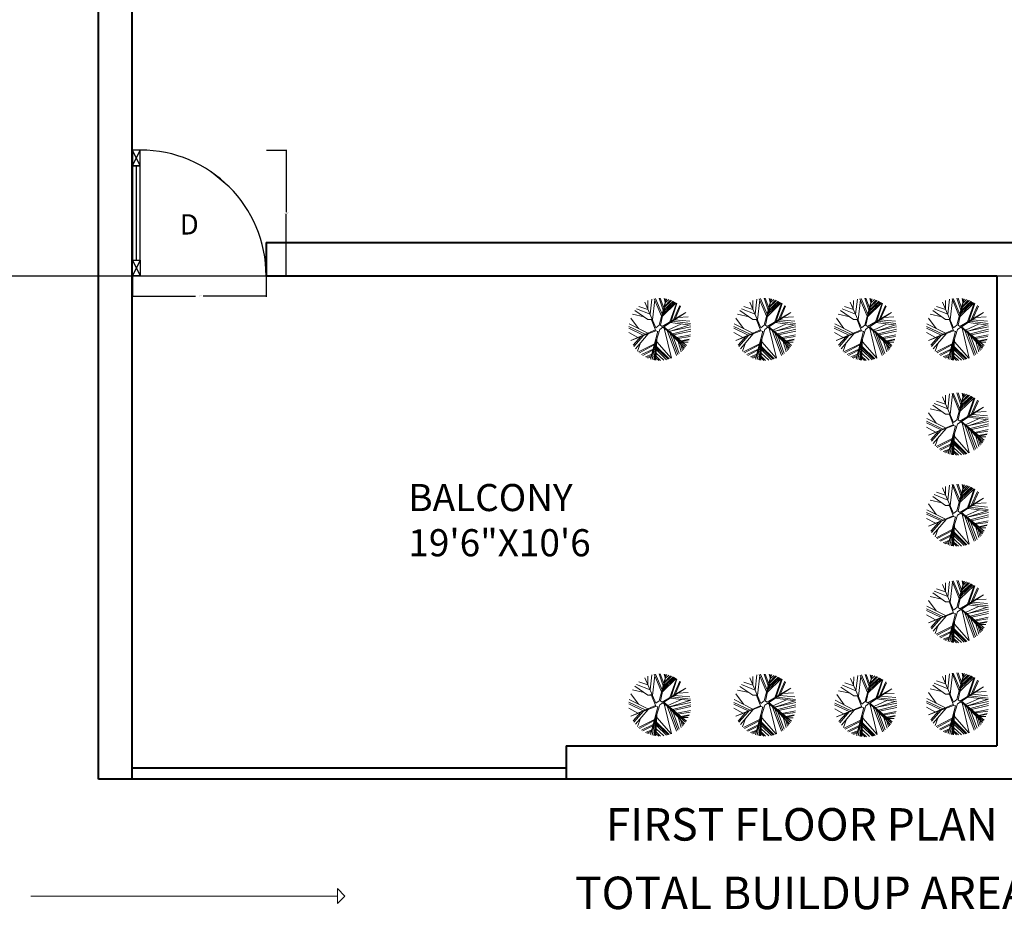
# Model space of a CAD drawing. Units: inches. Extents: x 182 to 1022, y -617 to 111.
# Tile 23 of 33: x 615 to 879, y -578 to -337. Entities that reach past the tile are written whole.
import ezdxf

# ---------------------------------------------------------------- set-up
doc = ezdxf.new("R2010")
doc.units = ezdxf.units.IN
doc.header["$MEASUREMENT"] = 0
for name, color, linetype, lineweight in [('A-ANNO-DIMS', 2, 'Continuous', 18), ('A-ANNO-IDEN', 1, 'Continuous', 18), ('A-ANNO-SYMB', 1, 'Continuous', 15), ('A-ANNO-TEXT', 8, 'Continuous', 20), ('A-AREA-IDEN', 8, 'Continuous', 18), ('door', 2, 'Continuous', 25), ('wall', 1, 'Continuous', 40)]:
    doc.layers.add(name, color=color, linetype=linetype, lineweight=lineweight)
doc.layers.add('GRASS', color=90, linetype='Continuous', lineweight=13, transparency=0.7)
doc.styles.get("Standard").update_dxf_attribs({"font": 'arial.ttf'})
doc.dimstyles.get("Standard").update_dxf_attribs({"dimtxt": 0.18, "dimasz": 0.18, "dimexe": 0.18, "dimexo": 0.0625, "dimgap": 0.09, "dimtad": 0, "dimtih": 1, "dimtoh": 1, "dimdec": 1, "dimzin": 0, "dimdsep": 46, "dimlunit": 4, "dimtxsty": 'Standard', "dimcen": 0.09, "dimadec": 0, "dimazin": 0, "dimtfac": 1, "dimtdec": 1, "dimtofl": 0, "dimtmove": 0, "dimatfit": 3, "dimfxl": 1, "dimtolj": 1, "dimtzin": 0, "dimarcsym": 0})

# ---------------------------------------------------------------- blocks, each defined once
blk = doc.blocks.new('A$C2D7661C6')
for p, q in [((0, 700), (50, 800)), ((50, 700), (0, 800)), ((25, 700), (25, 100)), ((50, 100), (0, 0)), ((0, 100), (50, 0))]:
    blk.add_line(p, q)
for points in [[(0, 700), (50, 700), (50, 800), (0, 800)], [(0, 100), (50, 100), (50, 700), (0, 700)], [(0, 100), (50, 100), (50, 0), (0, 0)]]:
    blk.add_lwpolyline(points, close=True)
blk.add_arc((50, 0), 800, 0, 90)
blk = doc.blocks.new('A$C7F556C88')
for p, q in [((615.7, 565.7), (500.3, 661.3)), ((50, 0), (850, 0))]:
    blk.add_line(p, q)
blk.add_blockref('A$C2D7661C6', (0, 0))
blk = doc.blocks.new('A$C4FA53466')
at = {"color": 0}
for p, q in [((0.501, 1.356), (0.505, 1.578)), ((0.563, 1.216), (0.612, 1.614)), ((0.627, 1.07), (0.687, 1.601)), ((0.867, 1.166), (0.675, 1.628)), ((0.882, 1.223), (0.709, 1.633)), ((0.91, 1.328), (0.802, 1.64)), ((0.988, 1.623), (0.804, 0.931)), ((0.925, 1.384), (0.834, 1.64)), ((0.836, 0.927), (0.988, 1.623)), ((0.922, 1.323), (1.176, 1.559)), ((0.964, 1.534), (0.938, 1.632)), ((0.938, 1.393), (1.132, 1.579)), ((0.945, 1.425), (1.104, 1.59)), ((0.967, 1.545), (0.952, 1.63)), ((0.965, 1.517), (1.059, 1.605)), ((0.974, 1.559), (1.002, 1.62)), ((0.506, 1.079), (0.165, 1.314)), ((0.562, 1.217), (0.205, 1.363)), ((0.505, 1.347), (0.266, 1.426)), ((0.717, 0.864), (0.422, 1.538)), ((0.887, 1.159), (1.256, 1.515)), ((0.901, 1.223), (1.228, 1.532)), ((0.914, 1.283), (1.197, 1.549)), ((1.085, 1.015), (1.262, 1.512)), ((1.121, 1.036), (1.274, 1.503)), ((1.18, 1.071), (1.349, 1.447)), ((1.222, 1.096), (1.37, 1.428)), ((0.255, 0.841), (0.055, 1.116)), ((0.406, 1.148), (0.102, 1.217)), ((0.614, 1.092), (0.506, 1.079)), ((0.604, 1.069), (0.506, 1.079)), ((0.715, 0.784), (0.604, 1.069)), ((1.509, 1.265), (0.879, 0.894)), ((0.926, 0.889), (1.509, 1.265)), ((1.211, 1.073), (1.612, 1.034)), ((1.3, 1.13), (1.573, 1.147)), ((0.384, 0.667), (0, 0.848)), ((0.436, 0.689), (0.003, 0.892)), ((0.501, 0.716), (0.012, 0.965)), ((0.053, 0.528), (0.708, 0.803)), ((0.716, 0.781), (0.053, 0.528)), ((0.82, 0.82), (0.575, 0.037)), ((0.715, 0.784), (0.775, 0.767)), ((0.804, 0.931), (0.717, 0.864)), ((0.82, 0.82), (0.904, 0.875)), ((0.879, 0.894), (0.836, 0.927)), ((1.521, 0.394), (0.904, 0.875)), ((0.926, 0.889), (1.521, 0.394)), ((0.938, 0.848), (1.126, 0.059)), ((1.016, 0.788), (1.263, 0.13)), ((1.03, 0.802), (1.392, 0.963)), ((1.073, 0.767), (1.614, 0.936)), ((1.081, 0.769), (1.638, 0.886)), ((1.097, 0.999), (1.632, 0.934)), ((1.148, 1.032), (1.626, 0.972)), ((1.153, 0.701), (1.64, 0.826)), ((0.237, 0.605), (0.004, 0.735)), ((0.321, 0.63), (0.115, 0.4)), ((0.387, 0.655), (0.137, 0.366)), ((0.516, 0.704), (0.179, 0.309)), ((0.575, 0.037), (0.769, 0.772)), ((0.732, 0.539), (0.664, 0.015)), ((0.737, 0.554), (0.691, 0.01)), ((0.744, 0.569), (0.717, 0.006)), ((1.04, 0.769), (1.475, 0.326)), ((1.06, 0.754), (1.5, 0.362)), ((1.083, 0.725), (1.298, 0.153)), ((1.161, 0.646), (1.335, 0.182)), ((1.185, 0.674), (1.639, 0.776)), ((1.273, 0.601), (1.627, 0.672)), ((1.298, 0.58), (1.618, 0.629)), ((1.376, 0.515), (1.599, 0.562)), ((1.392, 0.502), (1.593, 0.545)), ((0.313, 0.466), (0.232, 0.248)), ((0.682, 0.44), (0.255, 0.225)), ((0.673, 0.407), (0.281, 0.201)), ((0.645, 0.301), (0.342, 0.153)), ((0.636, 0.267), (0.375, 0.133)), ((0.701, 0.44), (0.621, 0.024)), ((0.73, 0.277), (0.998, 0.019)), ((0.733, 0.326), (1.037, 0.029)), ((0.735, 0.369), (1.067, 0.038)), ((0.74, 0.488), (1.121, 0.057)), ((1.301, 0.503), (1.386, 0.227)), ((1.365, 0.438), (1.42, 0.26)), ((1.412, 0.486), (1.569, 0.486)), ((1.413, 0.39), (1.444, 0.288)), ((0.608, 0.161), (0.439, 0.093)), ((0.6, 0.133), (0.475, 0.076)), ((0.59, 0.094), (0.501, 0.064)), ((0.72, 0.07), (0.793, 0)), ((0.722, 0.111), (0.842, 0)), ((0.726, 0.192), (0.924, 0.006))]:
    blk.add_line(p, q, dxfattribs=at)
blk = doc.blocks.new('*D14')
at = {"layer": 'A-ANNO-DIMS', "color": 0, "lineweight": -2, "transparency": 16777216}
for p, q in [((645.42, -405.44), (645.42, -410.94)), ((681.3, -405.44), (681.3, -410.94)), ((645.6, -410.76), (662.32, -410.76)), ((681.12, -410.76), (664.41, -410.76))]:
    blk.add_line(p, q, dxfattribs=at)
at = {"layer": 'A-ANNO-DIMS', "color": 0, "transparency": 16777216}
for points in [[(645.6, -410.73), (645.6, -410.79), (645.42, -410.76)], [(681.12, -410.73), (681.12, -410.79), (681.3, -410.76)]]:
    blk.add_solid(points, dxfattribs=at)
at = {"layer": 'Defpoints', "color": 0, "transparency": 16777216}
for p in [(645.42, -405.37), (681.3, -405.37), (681.3, -410.76)]:
    blk.add_point(p, dxfattribs=at)
at = {"layer": 'A-ANNO-DIMS', "color": 0, "transparency": 16777216, "insert": (663.36, -410.76), "char_height": 0.18, "attachment_point": 5}
blk.add_mtext('\\A1;DOOR 3\'-0" TYP.', dxfattribs=at)
blk = doc.blocks.new('*D15')
at = {"layer": 'A-ANNO-DIMS', "color": 0, "lineweight": -2, "transparency": 16777216}
for p, q in [((681.37, -371.6), (686.87, -371.6)), ((686.69, -371.78), (686.69, -388.31)), ((686.69, -405.19), (686.69, -388.67)), ((681.37, -405.37), (686.87, -405.37))]:
    blk.add_line(p, q, dxfattribs=at)
at = {"layer": 'A-ANNO-DIMS', "color": 0, "transparency": 16777216}
for points in [[(686.66, -371.78), (686.72, -371.78), (686.69, -371.6)], [(686.66, -405.19), (686.72, -405.19), (686.69, -405.37)]]:
    blk.add_solid(points, dxfattribs=at)
at = {"layer": 'Defpoints', "color": 0, "transparency": 16777216}
for p in [(681.3, -371.6), (686.69, -371.6), (681.3, -405.37)]:
    blk.add_point(p, dxfattribs=at)
at = {"layer": 'A-ANNO-DIMS', "color": 0, "transparency": 16777216, "insert": (686.69, -388.49), "char_height": 0.18, "attachment_point": 5}
blk.add_mtext('\\A1;2\'-10" TYP.', dxfattribs=at)
blk = doc.blocks.new('*D39')
at = {"layer": 'A-ANNO-DIMS', "color": 0, "lineweight": -2, "transparency": 16777216}
for p, q in [((238.4, -288.54), (1015.28, -288.54)), ((1015.1, -288.72), (1015.1, -346.77)), ((1015.1, -405.19), (1015.1, -347.14)), ((238.43, -405.37), (1015.28, -405.37))]:
    blk.add_line(p, q, dxfattribs=at)
at = {"layer": 'A-ANNO-DIMS', "color": 0, "transparency": 16777216}
for points in [[(1015.07, -288.72), (1015.13, -288.72), (1015.1, -288.54)], [(1015.07, -405.19), (1015.13, -405.19), (1015.1, -405.37)]]:
    blk.add_solid(points, dxfattribs=at)
at = {"layer": 'Defpoints', "color": 0, "transparency": 16777216}
for p in [(238.34, -288.54), (1015.1, -288.54), (238.36, -405.37)]:
    blk.add_point(p, dxfattribs=at)
at = {"layer": 'A-ANNO-DIMS', "color": 0, "transparency": 16777216, "insert": (1015.1, -346.96), "char_height": 0.18, "attachment_point": 5}
blk.add_mtext('\\A1;9\'-9"', dxfattribs=at)

msp = doc.modelspace()

# ---------------------------------------------------------------- linework, layer by layer
at = {"layer": 'A-ANNO-SYMB'}
for p, q in [((700.43, -571.69), (700.43, -569.69)), ((702.43, -571.69), (700.43, -569.69)), ((618.15, -571.69), (700.43, -571.69)), ((700.43, -571.69), (700.43, -573.69)), ((702.43, -571.69), (700.43, -573.69))]:
    msp.add_line(p, q, dxfattribs=at)
at = {"layer": 'wall'}
for p, q in [((636.3, -540.37), (636.3, -0.37)), ((645.3, -9.37), (645.3, -540.37)), ((681.3, -396.37), (881.3, -396.37)), ((681.3, -396.37), (681.3, -405.37)), ((681.3, -405.37), (877.3, -405.37)), ((877.3, -405.37), (877.3, -531.37)), ((761.8, -531.37), (877.3, -531.37)), ((761.8, -531.37), (761.8, -540.37)), ((761.8, -537.37), (645.3, -537.37)), ((972.3, -540.37), (636.3, -540.37))]:
    msp.add_line(p, q, dxfattribs=at)

# ---------------------------------------------------------------- block references
at = {"layer": 'door', "xscale": 0.042214023418219, "yscale": 0.042214023418219, "zscale": 0.042214023418219}
msp.add_blockref('A$C7F556C88', (645.42, -405.37), dxfattribs=at)
at = {"layer": 'GRASS', "xscale": 10.16810711056296, "yscale": 10.16810711056296, "zscale": 10.16810711056296}
for p in [(778.55, -428.03), (806.72, -428.03), (833.7, -428.03), (858.42, -428.03), (858.42, -453.43), (858.42, -477.87), (858.42, -503.76), (778.55, -528.77), (806.72, -528.81), (833.79, -528.98), (858.42, -528.48)]:
    msp.add_blockref('A$C4FA53466', p, dxfattribs=at)

# ---------------------------------------------------------------- texts
at = {"layer": 'A-ANNO-IDEN'}
msp.add_text('D', height=5.44, dxfattribs=at).set_placement((658.12, -394.26))
at = {"layer": 'A-ANNO-TEXT', "char_height": 8.7185, "attachment_point": 1}
for s, width, insert in [('FIRST FLOOR PLAN', 120.6589, (772.38, -548.1)), ('TOTAL BUILDUP AREA = 1260sqft', 195.6714, (764.16, -566.48))]:
    msp.add_mtext_dynamic_manual_height_columns(s, width=width, gutter_width=1.45, heights=[0], dxfattribs=dict(at, insert=insert))
at = {"layer": 'A-AREA-IDEN', "insert": (719.44, -461.17), "char_height": 7.2703, "attachment_point": 1}
msp.add_mtext_dynamic_manual_height_columns('BALCONY      19\'6"X10\'6', width=56.2356, gutter_width=1.21, heights=[0], dxfattribs=at)

# ---------------------------------------------------------------- dimensions: what is measured, and where the dimension line sits
at = {"layer": 'A-ANNO-DIMS'}
dim = msp.add_linear_dim(base=(1015.1, -288.54), p1=(238.36, -405.37), p2=(238.34, -288.54), angle=90, dimstyle='Standard', override={"dimdec": 1, "dimlfac": 1, "dimrnd": 0, "dimzin": 1, "dimdsep": 46, "dimlunit": 4, "dimfrac": 2}, dxfattribs=at)
dim.commit()
dim.dimension.update_dxf_attribs({"geometry": '*D39', "text_midpoint": (1015.1, -346.96)})
dim = msp.add_linear_dim(base=(686.69, -371.6), p1=(681.3, -405.37), p2=(681.3, -371.6), angle=90, text='<> TYP.', dimstyle='Standard', override={"dimdec": 1, "dimlfac": 1, "dimrnd": 0, "dimzin": 1, "dimdsep": 46, "dimlunit": 4, "dimfrac": 2}, dxfattribs=at)
dim.commit()
dim.dimension.update_dxf_attribs({"geometry": '*D15', "text_midpoint": (686.69, -388.49)})
dim = msp.add_linear_dim(base=(681.3, -410.76), p1=(645.42, -405.37), p2=(681.3, -405.37), text='DOOR <> TYP.', dimstyle='Standard', override={"dimdec": 1, "dimlfac": 1, "dimrnd": 0, "dimzin": 1, "dimdsep": 46, "dimlunit": 4, "dimfrac": 2}, dxfattribs=at)
dim.commit()
dim.dimension.update_dxf_attribs({"geometry": '*D14', "text_midpoint": (663.36, -410.76)})

doc.saveas('drawing.dxf')
